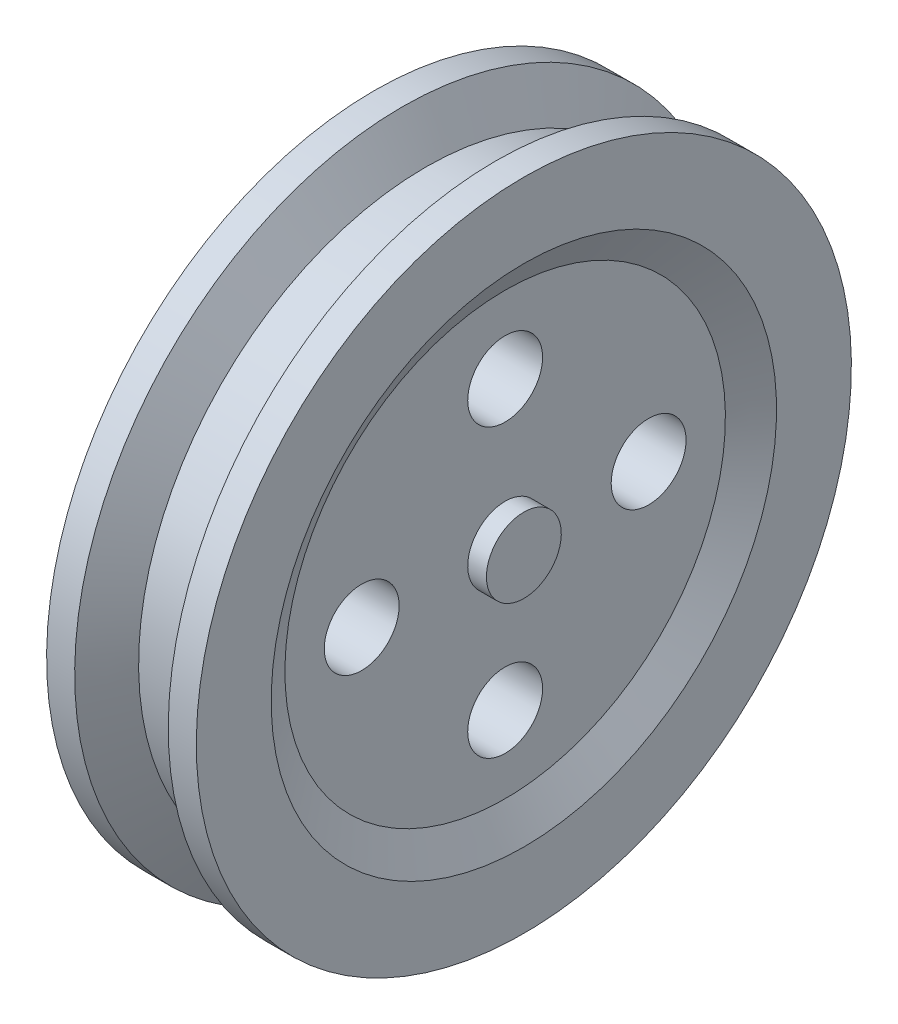
ISO-10303-21;
HEADER;
FILE_DESCRIPTION(('STEP AP214'),'2;1');
FILE_NAME('part.step','',(''),(''),'','','');
FILE_SCHEMA(('AUTOMOTIVE_DESIGN { 1 0 10303 214 1 1 1 1 }'));
ENDSEC;
DATA;
#1=APPLICATION_CONTEXT('core data for automotive mechanical design processes');
#2=APPLICATION_PROTOCOL_DEFINITION('international standard','automotive_design',2000,#1);
#3=PRODUCT_CONTEXT('',#1,'mechanical');
#4=PRODUCT('Part','Part','',(#3));
#5=PRODUCT_RELATED_PRODUCT_CATEGORY('part','',(#4));
#6=PRODUCT_DEFINITION_FORMATION('','',#4);
#7=PRODUCT_DEFINITION_CONTEXT('part definition',#1,'design');
#8=PRODUCT_DEFINITION('design','',#6,#7);
#9=PRODUCT_DEFINITION_SHAPE('','',#8);
#10=(LENGTH_UNIT() NAMED_UNIT(*) SI_UNIT(.MILLI.,.METRE.));
#11=(NAMED_UNIT(*) PLANE_ANGLE_UNIT() SI_UNIT($,.RADIAN.));
#12=(NAMED_UNIT(*) SI_UNIT($,.STERADIAN.) SOLID_ANGLE_UNIT());
#13=UNCERTAINTY_MEASURE_WITH_UNIT(LENGTH_MEASURE(1.E-05),#10,'distance_accuracy_value','');
#14=(GEOMETRIC_REPRESENTATION_CONTEXT(3) GLOBAL_UNCERTAINTY_ASSIGNED_CONTEXT((#13)) GLOBAL_UNIT_ASSIGNED_CONTEXT((#10,
#11,#12)) REPRESENTATION_CONTEXT('',''));
#15=CARTESIAN_POINT('',(0.,0.,0.));
#16=DIRECTION('',(0.,0.,1.));
#17=DIRECTION('',(1.,0.,0.));
#18=AXIS2_PLACEMENT_3D('',#15,#16,#17);
#19=CARTESIAN_POINT('',(8.,6.,0.));
#20=DIRECTION('',(1.,0.,0.));
#21=DIRECTION('',(0.,1.,0.));
#22=AXIS2_PLACEMENT_3D('',#19,#20,#21);
#23=CYLINDRICAL_SURFACE('',#22,4.);
#24=CARTESIAN_POINT('',(6.,6.,0.));
#25=DIRECTION('',(1.,0.,0.));
#26=DIRECTION('',(0.,1.,0.));
#27=AXIS2_PLACEMENT_3D('',#24,#25,#26);
#28=CIRCLE('',#27,4.);
#29=CARTESIAN_POINT('',(6.,10.,0.));
#30=VERTEX_POINT('',#29);
#31=EDGE_CURVE('E63',#30,#30,#28,.T.);
#32=ORIENTED_EDGE('',*,*,#31,.T.);
#33=EDGE_LOOP('',(#32));
#34=FACE_BOUND('',#33,.T.);
#35=CARTESIAN_POINT('',(8.,6.,0.));
#36=DIRECTION('',(1.,0.,0.));
#37=DIRECTION('',(0.,1.,0.));
#38=AXIS2_PLACEMENT_3D('',#35,#36,#37);
#39=CIRCLE('',#38,4.);
#40=CARTESIAN_POINT('',(8.,10.,0.));
#41=VERTEX_POINT('',#40);
#42=EDGE_CURVE('E10',#41,#41,#39,.T.);
#43=ORIENTED_EDGE('',*,*,#42,.F.);
#44=EDGE_LOOP('',(#43));
#45=FACE_BOUND('',#44,.T.);
#46=ADVANCED_FACE('F40',(#34,#45),#23,.T.);
#47=CARTESIAN_POINT('',(8.,6.,0.));
#48=DIRECTION('',(1.,0.,0.));
#49=DIRECTION('',(0.,1.,0.));
#50=AXIS2_PLACEMENT_3D('',#47,#48,#49);
#51=PLANE('',#50);
#52=ORIENTED_EDGE('',*,*,#42,.T.);
#53=EDGE_LOOP('',(#52));
#54=FACE_BOUND('',#53,.T.);
#55=ADVANCED_FACE('F123',(#54),#51,.T.);
#56=CARTESIAN_POINT('',(-8.,6.,0.));
#57=DIRECTION('',(-1.,0.,0.));
#58=DIRECTION('',(0.,-1.,0.));
#59=AXIS2_PLACEMENT_3D('',#56,#57,#58);
#60=PLANE('',#59);
#61=CARTESIAN_POINT('',(-8.,6.,0.));
#62=DIRECTION('',(1.,0.,0.));
#63=DIRECTION('',(0.,1.,0.));
#64=AXIS2_PLACEMENT_3D('',#61,#62,#63);
#65=CIRCLE('',#64,4.);
#66=CARTESIAN_POINT('',(-8.,10.,0.));
#67=VERTEX_POINT('',#66);
#68=EDGE_CURVE('E42',#67,#67,#65,.T.);
#69=ORIENTED_EDGE('',*,*,#68,.F.);
#70=EDGE_LOOP('',(#69));
#71=FACE_BOUND('',#70,.T.);
#72=ADVANCED_FACE('F115',(#71),#60,.T.);
#73=CARTESIAN_POINT('',(8.,6.,0.));
#74=DIRECTION('',(1.,0.,0.));
#75=DIRECTION('',(0.,1.,0.));
#76=AXIS2_PLACEMENT_3D('',#73,#74,#75);
#77=CYLINDRICAL_SURFACE('',#76,4.);
#78=ORIENTED_EDGE('',*,*,#68,.T.);
#79=EDGE_LOOP('',(#78));
#80=FACE_BOUND('',#79,.T.);
#81=CARTESIAN_POINT('',(-6.,6.,0.));
#82=DIRECTION('',(1.,0.,0.));
#83=DIRECTION('',(0.,1.,0.));
#84=AXIS2_PLACEMENT_3D('',#81,#82,#83);
#85=CIRCLE('',#84,4.);
#86=CARTESIAN_POINT('',(-6.,10.,0.));
#87=VERTEX_POINT('',#86);
#88=EDGE_CURVE('E47',#87,#87,#85,.T.);
#89=ORIENTED_EDGE('',*,*,#88,.F.);
#90=EDGE_LOOP('',(#89));
#91=FACE_BOUND('',#90,.T.);
#92=ADVANCED_FACE('F109',(#80,#91),#77,.T.);
#93=CARTESIAN_POINT('',(-6.,10.,0.));
#94=DIRECTION('',(-1.,0.,0.));
#95=DIRECTION('',(0.,-1.,0.));
#96=AXIS2_PLACEMENT_3D('',#93,#94,#95);
#97=PLANE('',#96);
#98=CARTESIAN_POINT('',(-6.,21.3295637837594,0.));
#99=DIRECTION('',(-1.,0.,0.));
#100=DIRECTION('',(0.,-1.,0.));
#101=AXIS2_PLACEMENT_3D('',#98,#99,#100);
#102=CIRCLE('',#101,4.);
#103=CARTESIAN_POINT('',(-6.,17.3295637837594,0.));
#104=VERTEX_POINT('',#103);
#105=EDGE_CURVE('E60',#104,#104,#102,.T.);
#106=ORIENTED_EDGE('',*,*,#105,.F.);
#107=EDGE_LOOP('',(#106));
#108=FACE_BOUND('',#107,.T.);
#109=CARTESIAN_POINT('',(-6.,6.,-15.3295637837594));
#110=DIRECTION('',(-1.,0.,0.));
#111=DIRECTION('',(0.,-1.,0.));
#112=AXIS2_PLACEMENT_3D('',#109,#110,#111);
#113=CIRCLE('',#112,4.);
#114=CARTESIAN_POINT('',(-6.,2.,-15.3295637837594));
#115=VERTEX_POINT('',#114);
#116=EDGE_CURVE('E292',#115,#115,#113,.T.);
#117=ORIENTED_EDGE('',*,*,#116,.F.);
#118=EDGE_LOOP('',(#117));
#119=FACE_BOUND('',#118,.T.);
#120=CARTESIAN_POINT('',(-6.,6.,15.3295637837594));
#121=DIRECTION('',(-1.,0.,0.));
#122=DIRECTION('',(0.,-1.,0.));
#123=AXIS2_PLACEMENT_3D('',#120,#121,#122);
#124=CIRCLE('',#123,4.);
#125=CARTESIAN_POINT('',(-6.,2.,15.3295637837594));
#126=VERTEX_POINT('',#125);
#127=EDGE_CURVE('E294',#126,#126,#124,.T.);
#128=ORIENTED_EDGE('',*,*,#127,.F.);
#129=EDGE_LOOP('',(#128));
#130=FACE_BOUND('',#129,.T.);
#131=CARTESIAN_POINT('',(-6.,-9.3295637837594,0.));
#132=DIRECTION('',(-1.,0.,0.));
#133=DIRECTION('',(0.,-1.,0.));
#134=AXIS2_PLACEMENT_3D('',#131,#132,#133);
#135=CIRCLE('',#134,4.);
#136=CARTESIAN_POINT('',(-6.,-13.3295637837594,0.));
#137=VERTEX_POINT('',#136);
#138=EDGE_CURVE('E79',#137,#137,#135,.T.);
#139=ORIENTED_EDGE('',*,*,#138,.F.);
#140=EDGE_LOOP('',(#139));
#141=FACE_BOUND('',#140,.T.);
#142=ORIENTED_EDGE('',*,*,#88,.T.);
#143=EDGE_LOOP('',(#142));
#144=FACE_BOUND('',#143,.T.);
#145=CARTESIAN_POINT('',(-6.,6.,0.));
#146=DIRECTION('',(1.,0.,0.));
#147=DIRECTION('',(0.,1.,0.));
#148=AXIS2_PLACEMENT_3D('',#145,#146,#147);
#149=CIRCLE('',#148,23.5358983848623);
#150=CARTESIAN_POINT('',(-6.,29.5358983848623,0.));
#151=VERTEX_POINT('',#150);
#152=EDGE_CURVE('E105',#151,#151,#149,.T.);
#153=ORIENTED_EDGE('',*,*,#152,.F.);
#154=EDGE_LOOP('',(#153));
#155=FACE_BOUND('',#154,.T.);
#156=ADVANCED_FACE('F110',(#108,#119,#130,#141,#144,#155),#97,.T.);
#157=CARTESIAN_POINT('',(-7.99999999999999,6.,0.));
#158=DIRECTION('',(-1.,0.,0.));
#159=DIRECTION('',(0.,-1.,0.));
#160=AXIS2_PLACEMENT_3D('',#157,#158,#159);
#161=CONICAL_SURFACE('',#160,27.,1.0471975511966);
#162=ORIENTED_EDGE('',*,*,#152,.T.);
#163=EDGE_LOOP('',(#162));
#164=FACE_BOUND('',#163,.T.);
#165=CARTESIAN_POINT('',(-7.99999999999999,6.,0.));
#166=DIRECTION('',(1.,0.,0.));
#167=DIRECTION('',(0.,1.,0.));
#168=AXIS2_PLACEMENT_3D('',#165,#166,#167);
#169=CIRCLE('',#168,27.);
#170=CARTESIAN_POINT('',(-8.,33.,0.));
#171=VERTEX_POINT('',#170);
#172=EDGE_CURVE('E97',#171,#171,#169,.T.);
#173=ORIENTED_EDGE('',*,*,#172,.F.);
#174=EDGE_LOOP('',(#173));
#175=FACE_BOUND('',#174,.T.);
#176=ADVANCED_FACE('F117',(#164,#175),#161,.F.);
#177=CARTESIAN_POINT('',(-8.,33.,0.));
#178=DIRECTION('',(-1.,0.,0.));
#179=DIRECTION('',(0.,-1.,0.));
#180=AXIS2_PLACEMENT_3D('',#177,#178,#179);
#181=PLANE('',#180);
#182=ORIENTED_EDGE('',*,*,#172,.T.);
#183=EDGE_LOOP('',(#182));
#184=FACE_BOUND('',#183,.T.);
#185=CARTESIAN_POINT('',(-7.99999999999999,6.,0.));
#186=DIRECTION('',(1.,0.,0.));
#187=DIRECTION('',(0.,1.,0.));
#188=AXIS2_PLACEMENT_3D('',#185,#186,#187);
#189=CIRCLE('',#188,35.);
#190=CARTESIAN_POINT('',(-8.,41.,0.));
#191=VERTEX_POINT('',#190);
#192=EDGE_CURVE('E96',#191,#191,#189,.T.);
#193=ORIENTED_EDGE('',*,*,#192,.F.);
#194=EDGE_LOOP('',(#193));
#195=FACE_BOUND('',#194,.T.);
#196=ADVANCED_FACE('F157',(#184,#195),#181,.T.);
#197=CARTESIAN_POINT('',(8.,6.,0.));
#198=DIRECTION('',(1.,0.,0.));
#199=DIRECTION('',(0.,1.,0.));
#200=AXIS2_PLACEMENT_3D('',#197,#198,#199);
#201=CYLINDRICAL_SURFACE('',#200,35.);
#202=ORIENTED_EDGE('',*,*,#192,.T.);
#203=EDGE_LOOP('',(#202));
#204=FACE_BOUND('',#203,.T.);
#205=CARTESIAN_POINT('',(-5.00000000000001,6.,0.));
#206=DIRECTION('',(1.,0.,0.));
#207=DIRECTION('',(0.,1.,0.));
#208=AXIS2_PLACEMENT_3D('',#205,#206,#207);
#209=CIRCLE('',#208,35.);
#210=CARTESIAN_POINT('',(-5.00000000000002,41.,0.));
#211=VERTEX_POINT('',#210);
#212=EDGE_CURVE('E91',#211,#211,#209,.T.);
#213=ORIENTED_EDGE('',*,*,#212,.F.);
#214=EDGE_LOOP('',(#213));
#215=FACE_BOUND('',#214,.T.);
#216=ADVANCED_FACE('F166',(#204,#215),#201,.T.);
#217=CARTESIAN_POINT('',(-2.50000000000001,6.,0.));
#218=DIRECTION('',(-1.,0.,0.));
#219=DIRECTION('',(0.,-1.,0.));
#220=AXIS2_PLACEMENT_3D('',#217,#218,#219);
#221=CONICAL_SURFACE('',#220,30.6698729810778,1.0471975511966);
#222=ORIENTED_EDGE('',*,*,#212,.T.);
#223=EDGE_LOOP('',(#222));
#224=FACE_BOUND('',#223,.T.);
#225=CARTESIAN_POINT('',(-2.50000000000001,6.,0.));
#226=DIRECTION('',(1.,0.,0.));
#227=DIRECTION('',(0.,1.,0.));
#228=AXIS2_PLACEMENT_3D('',#225,#226,#227);
#229=CIRCLE('',#228,30.6698729810778);
#230=CARTESIAN_POINT('',(-2.50000000000001,36.6698729810778,0.));
#231=VERTEX_POINT('',#230);
#232=EDGE_CURVE('E89',#231,#231,#229,.T.);
#233=ORIENTED_EDGE('',*,*,#232,.F.);
#234=EDGE_LOOP('',(#233));
#235=FACE_BOUND('',#234,.T.);
#236=ADVANCED_FACE('F177',(#224,#235),#221,.T.);
#237=CARTESIAN_POINT('',(8.,6.,0.));
#238=DIRECTION('',(1.,0.,0.));
#239=DIRECTION('',(0.,1.,0.));
#240=AXIS2_PLACEMENT_3D('',#237,#238,#239);
#241=CYLINDRICAL_SURFACE('',#240,30.6698729810778);
#242=ORIENTED_EDGE('',*,*,#232,.T.);
#243=EDGE_LOOP('',(#242));
#244=FACE_BOUND('',#243,.T.);
#245=CARTESIAN_POINT('',(2.49999999999999,6.,0.));
#246=DIRECTION('',(1.,0.,0.));
#247=DIRECTION('',(0.,1.,0.));
#248=AXIS2_PLACEMENT_3D('',#245,#246,#247);
#249=CIRCLE('',#248,30.6698729810778);
#250=CARTESIAN_POINT('',(2.49999999999999,36.6698729810778,0.));
#251=VERTEX_POINT('',#250);
#252=EDGE_CURVE('E87',#251,#251,#249,.T.);
#253=ORIENTED_EDGE('',*,*,#252,.F.);
#254=EDGE_LOOP('',(#253));
#255=FACE_BOUND('',#254,.T.);
#256=ADVANCED_FACE('F188',(#244,#255),#241,.T.);
#257=CARTESIAN_POINT('',(5.,6.,0.));
#258=DIRECTION('',(1.,0.,0.));
#259=DIRECTION('',(0.,1.,0.));
#260=AXIS2_PLACEMENT_3D('',#257,#258,#259);
#261=CONICAL_SURFACE('',#260,35.,1.0471975511966);
#262=ORIENTED_EDGE('',*,*,#252,.T.);
#263=EDGE_LOOP('',(#262));
#264=FACE_BOUND('',#263,.T.);
#265=CARTESIAN_POINT('',(5.,6.,0.));
#266=DIRECTION('',(1.,0.,0.));
#267=DIRECTION('',(0.,1.,0.));
#268=AXIS2_PLACEMENT_3D('',#265,#266,#267);
#269=CIRCLE('',#268,35.);
#270=CARTESIAN_POINT('',(4.99999999999999,41.,0.));
#271=VERTEX_POINT('',#270);
#272=EDGE_CURVE('E82',#271,#271,#269,.T.);
#273=ORIENTED_EDGE('',*,*,#272,.F.);
#274=EDGE_LOOP('',(#273));
#275=FACE_BOUND('',#274,.T.);
#276=ADVANCED_FACE('F200',(#264,#275),#261,.T.);
#277=CARTESIAN_POINT('',(8.,6.,0.));
#278=DIRECTION('',(1.,0.,0.));
#279=DIRECTION('',(0.,1.,0.));
#280=AXIS2_PLACEMENT_3D('',#277,#278,#279);
#281=CYLINDRICAL_SURFACE('',#280,35.);
#282=ORIENTED_EDGE('',*,*,#272,.T.);
#283=EDGE_LOOP('',(#282));
#284=FACE_BOUND('',#283,.T.);
#285=CARTESIAN_POINT('',(8.00000000000001,6.,0.));
#286=DIRECTION('',(1.,0.,0.));
#287=DIRECTION('',(0.,1.,0.));
#288=AXIS2_PLACEMENT_3D('',#285,#286,#287);
#289=CIRCLE('',#288,35.);
#290=CARTESIAN_POINT('',(8.,41.,0.));
#291=VERTEX_POINT('',#290);
#292=EDGE_CURVE('E81',#291,#291,#289,.T.);
#293=ORIENTED_EDGE('',*,*,#292,.F.);
#294=EDGE_LOOP('',(#293));
#295=FACE_BOUND('',#294,.T.);
#296=ADVANCED_FACE('F207',(#284,#295),#281,.T.);
#297=CARTESIAN_POINT('',(8.,33.,0.));
#298=DIRECTION('',(1.,0.,0.));
#299=DIRECTION('',(0.,1.,0.));
#300=AXIS2_PLACEMENT_3D('',#297,#298,#299);
#301=PLANE('',#300);
#302=ORIENTED_EDGE('',*,*,#292,.T.);
#303=EDGE_LOOP('',(#302));
#304=FACE_BOUND('',#303,.T.);
#305=CARTESIAN_POINT('',(8.00000000000001,6.,0.));
#306=DIRECTION('',(1.,0.,0.));
#307=DIRECTION('',(0.,1.,0.));
#308=AXIS2_PLACEMENT_3D('',#305,#306,#307);
#309=CIRCLE('',#308,27.);
#310=CARTESIAN_POINT('',(8.,33.,0.));
#311=VERTEX_POINT('',#310);
#312=EDGE_CURVE('E71',#311,#311,#309,.T.);
#313=ORIENTED_EDGE('',*,*,#312,.F.);
#314=EDGE_LOOP('',(#313));
#315=FACE_BOUND('',#314,.T.);
#316=ADVANCED_FACE('F218',(#304,#315),#301,.T.);
#317=CARTESIAN_POINT('',(6.,6.,0.));
#318=DIRECTION('',(1.,0.,0.));
#319=DIRECTION('',(0.,1.,0.));
#320=AXIS2_PLACEMENT_3D('',#317,#318,#319);
#321=CONICAL_SURFACE('',#320,23.5358983848623,1.04719755119659);
#322=ORIENTED_EDGE('',*,*,#312,.T.);
#323=EDGE_LOOP('',(#322));
#324=FACE_BOUND('',#323,.T.);
#325=CARTESIAN_POINT('',(6.,6.,0.));
#326=DIRECTION('',(1.,0.,0.));
#327=DIRECTION('',(0.,1.,0.));
#328=AXIS2_PLACEMENT_3D('',#325,#326,#327);
#329=CIRCLE('',#328,23.5358983848623);
#330=CARTESIAN_POINT('',(6.,29.5358983848623,0.));
#331=VERTEX_POINT('',#330);
#332=EDGE_CURVE('E68',#331,#331,#329,.T.);
#333=ORIENTED_EDGE('',*,*,#332,.F.);
#334=EDGE_LOOP('',(#333));
#335=FACE_BOUND('',#334,.T.);
#336=ADVANCED_FACE('F228',(#324,#335),#321,.F.);
#337=CARTESIAN_POINT('',(6.,10.,0.));
#338=DIRECTION('',(1.,0.,0.));
#339=DIRECTION('',(0.,1.,0.));
#340=AXIS2_PLACEMENT_3D('',#337,#338,#339);
#341=PLANE('',#340);
#342=CARTESIAN_POINT('',(6.,21.3295637837594,0.));
#343=DIRECTION('',(1.,0.,0.));
#344=DIRECTION('',(0.,1.,0.));
#345=AXIS2_PLACEMENT_3D('',#342,#343,#344);
#346=CIRCLE('',#345,4.);
#347=CARTESIAN_POINT('',(6.,25.3295637837594,0.));
#348=VERTEX_POINT('',#347);
#349=EDGE_CURVE('E37',#348,#348,#346,.T.);
#350=ORIENTED_EDGE('',*,*,#349,.F.);
#351=EDGE_LOOP('',(#350));
#352=FACE_BOUND('',#351,.T.);
#353=CARTESIAN_POINT('',(6.,6.,-15.3295637837594));
#354=DIRECTION('',(1.,0.,0.));
#355=DIRECTION('',(0.,1.,0.));
#356=AXIS2_PLACEMENT_3D('',#353,#354,#355);
#357=CIRCLE('',#356,4.);
#358=CARTESIAN_POINT('',(6.,10.,-15.3295637837594));
#359=VERTEX_POINT('',#358);
#360=EDGE_CURVE('E56',#359,#359,#357,.T.);
#361=ORIENTED_EDGE('',*,*,#360,.F.);
#362=EDGE_LOOP('',(#361));
#363=FACE_BOUND('',#362,.T.);
#364=CARTESIAN_POINT('',(6.,6.,15.3295637837594));
#365=DIRECTION('',(1.,0.,0.));
#366=DIRECTION('',(0.,1.,0.));
#367=AXIS2_PLACEMENT_3D('',#364,#365,#366);
#368=CIRCLE('',#367,4.);
#369=CARTESIAN_POINT('',(6.,10.,15.3295637837594));
#370=VERTEX_POINT('',#369);
#371=EDGE_CURVE('E57',#370,#370,#368,.T.);
#372=ORIENTED_EDGE('',*,*,#371,.F.);
#373=EDGE_LOOP('',(#372));
#374=FACE_BOUND('',#373,.T.);
#375=CARTESIAN_POINT('',(6.,-9.3295637837594,0.));
#376=DIRECTION('',(1.,0.,0.));
#377=DIRECTION('',(0.,1.,0.));
#378=AXIS2_PLACEMENT_3D('',#375,#376,#377);
#379=CIRCLE('',#378,4.);
#380=CARTESIAN_POINT('',(6.,-5.3295637837594,0.));
#381=VERTEX_POINT('',#380);
#382=EDGE_CURVE('E52',#381,#381,#379,.T.);
#383=ORIENTED_EDGE('',*,*,#382,.F.);
#384=EDGE_LOOP('',(#383));
#385=FACE_BOUND('',#384,.T.);
#386=ORIENTED_EDGE('',*,*,#332,.T.);
#387=EDGE_LOOP('',(#386));
#388=FACE_BOUND('',#387,.T.);
#389=ORIENTED_EDGE('',*,*,#31,.F.);
#390=EDGE_LOOP('',(#389));
#391=FACE_BOUND('',#390,.T.);
#392=ADVANCED_FACE('F236',(#352,#363,#374,#385,#388,#391),#341,.T.);
#393=CARTESIAN_POINT('',(8.00000000000001,-9.3295637837594,0.));
#394=DIRECTION('',(-1.,0.,0.));
#395=DIRECTION('',(0.,-1.,0.));
#396=AXIS2_PLACEMENT_3D('',#393,#394,#395);
#397=CYLINDRICAL_SURFACE('',#396,4.);
#398=ORIENTED_EDGE('',*,*,#382,.T.);
#399=EDGE_LOOP('',(#398));
#400=FACE_BOUND('',#399,.T.);
#401=ORIENTED_EDGE('',*,*,#138,.T.);
#402=EDGE_LOOP('',(#401));
#403=FACE_BOUND('',#402,.T.);
#404=ADVANCED_FACE('F250',(#400,#403),#397,.F.);
#405=CARTESIAN_POINT('',(8.00000000000001,6.,15.3295637837594));
#406=DIRECTION('',(-1.,0.,0.));
#407=DIRECTION('',(0.,-1.,0.));
#408=AXIS2_PLACEMENT_3D('',#405,#406,#407);
#409=CYLINDRICAL_SURFACE('',#408,4.);
#410=ORIENTED_EDGE('',*,*,#371,.T.);
#411=EDGE_LOOP('',(#410));
#412=FACE_BOUND('',#411,.T.);
#413=ORIENTED_EDGE('',*,*,#127,.T.);
#414=EDGE_LOOP('',(#413));
#415=FACE_BOUND('',#414,.T.);
#416=ADVANCED_FACE('F260',(#412,#415),#409,.F.);
#417=CARTESIAN_POINT('',(8.00000000000001,6.,-15.3295637837594));
#418=DIRECTION('',(-1.,0.,0.));
#419=DIRECTION('',(0.,-1.,0.));
#420=AXIS2_PLACEMENT_3D('',#417,#418,#419);
#421=CYLINDRICAL_SURFACE('',#420,4.);
#422=ORIENTED_EDGE('',*,*,#360,.T.);
#423=EDGE_LOOP('',(#422));
#424=FACE_BOUND('',#423,.T.);
#425=ORIENTED_EDGE('',*,*,#116,.T.);
#426=EDGE_LOOP('',(#425));
#427=FACE_BOUND('',#426,.T.);
#428=ADVANCED_FACE('F270',(#424,#427),#421,.F.);
#429=CARTESIAN_POINT('',(8.00000000000001,21.3295637837594,0.));
#430=DIRECTION('',(-1.,0.,0.));
#431=DIRECTION('',(0.,-1.,0.));
#432=AXIS2_PLACEMENT_3D('',#429,#430,#431);
#433=CYLINDRICAL_SURFACE('',#432,4.);
#434=ORIENTED_EDGE('',*,*,#349,.T.);
#435=EDGE_LOOP('',(#434));
#436=FACE_BOUND('',#435,.T.);
#437=ORIENTED_EDGE('',*,*,#105,.T.);
#438=EDGE_LOOP('',(#437));
#439=FACE_BOUND('',#438,.T.);
#440=ADVANCED_FACE('F280',(#436,#439),#433,.F.);
#441=CLOSED_SHELL('',(#46,#55,#72,#92,#156,#176,#196,#216,#236,#256,#276,#296,#316,#336,#392,
#404,#416,#428,#440));
#442=MANIFOLD_SOLID_BREP('B2',#441);
#443=ADVANCED_BREP_SHAPE_REPRESENTATION('',(#18,#442),#14);
#444=SHAPE_DEFINITION_REPRESENTATION(#9,#443);
ENDSEC;
END-ISO-10303-21;
